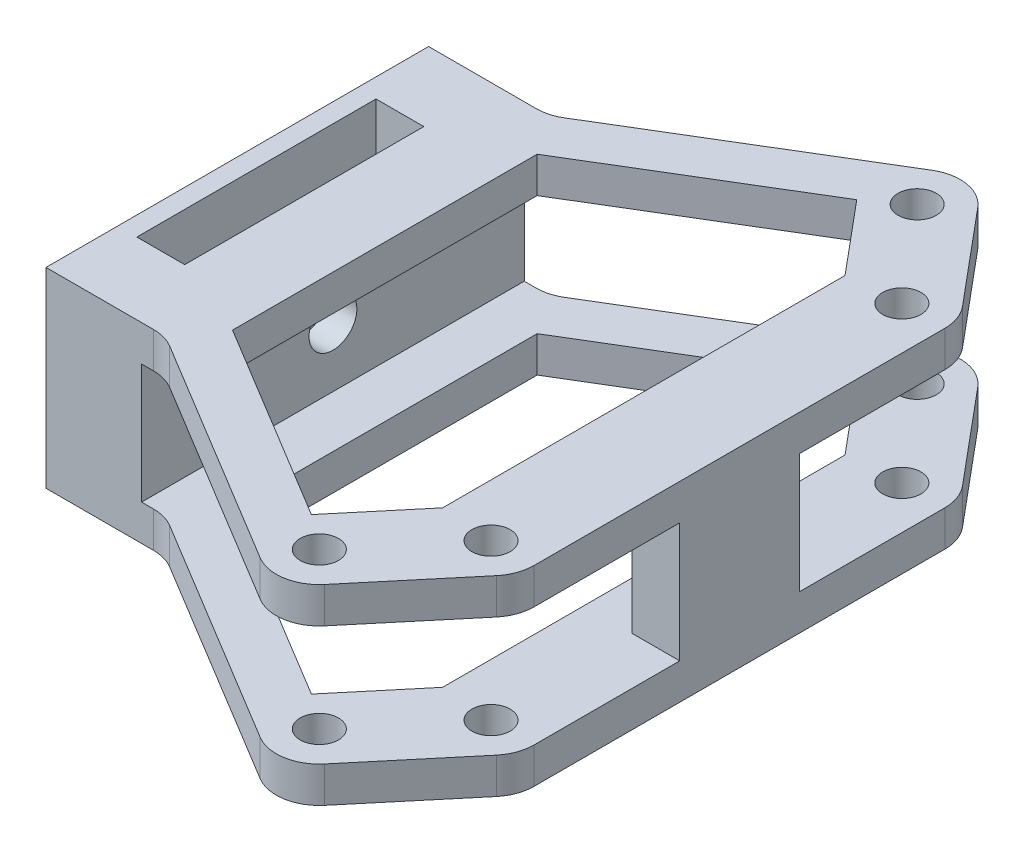
SolidWorks part; units mm, degrees
material "Plain Carbon Steel"
ref_plane "Front Plane" through (0, 0, 0) normal (0, 0, 1) x (1, 0, 0)
ref_plane "Top Plane" through (0, 0, 0) normal (0, 1, 0) x (1, 0, 0)
ref_plane "Right Plane" through (0, 0, 0) normal (1, 0, 0) x (0, 0, -1)
sketch "Frame Profile Sketch" plane through (0, 0, 0) normal (0, 1, 0) x (1, 0, 0)
  line L0 (-1085.7757, 0) -> (53203.0111, 0) construction
  line L1 (0, -1085.7757) -> (0, 53203.0111) construction
  line L2 (25, 40) -> (74.9963, 70.2034)
  line L3 (0, 40) -> (25, 40)
  line L4 (0, 40) -> (0, -40)
  line L5 (0, -40) -> (25, -40)
  line L7 (86.5538, 68.2738) -> (102.9038, 48.7238)
  line L8 (105, 42.95) -> (105, -42.95)
  line L9 (102.9038, -48.7238) -> (86.5538, -68.2738)
  line L10 (74.9963, -70.2034) -> (25, -40)
  arc A0 (102.9038, 48.7238) -> (105, 42.95) centre (96, 42.95) cw
  arc A1 (105, -42.95) -> (102.9038, -48.7238) centre (96, -42.95) cw
  arc A2 (86.5538, 68.2738) -> (74.9963, 70.2034) centre (79.65, 62.5) ccw
  arc A3 (86.5538, -68.2738) -> (74.9963, -70.2034) centre (79.65, -62.5) cw
  dimension "D5" = 9
  dimension "D1" = 80
  dimension "D2" = 25
  dimension "D3" = 40
  dimension "D4" = 105
  dimension "D6" = 16.35
  dimension "D7" = 16.35
  dimension "D8" = 85.9
  dimension "D9" = 42.95
  dimension "D10" = 19.55
  dimension "D11" = 19.55
  dimension "D12" = 25
extrude "Frame Body" add sketch "Frame Profile Sketch" along normal mid plane 40
sketch "Window and Holes Sketch" plane through (0, 0, 0) normal (0, 1, 0) x (1, 0, 0)
  line L0 (0, -1000) -> (0, 49000) construction
  line L1 (74.9963, 70.2034) -> (25, 40) construction
  line L2 (-1000, 0) -> (49000, 0) construction
  line L3 (30.85, 31.8509) -> (30.85, -31.8509)
  line L4 (4, 25) -> (14, 25)
  line L5 (4, 25) -> (4, -25)
  line L6 (4, -25) -> (14, -25)
  line L7 (14, 25) -> (14, -25)
  line L8 (30.85, -31.8509) -> (72.5046, -57.015)
  line L9 (72.5046, -57.015) -> (85, -42.074)
  line L10 (85, -42.074) -> (85, 42.074)
  line L11 (85, 42.074) -> (72.5046, 57.015)
  line L12 (72.5046, 57.015) -> (30.85, 31.8509)
  line L13 (25, -40) -> (74.9963, -70.2034) construction
  line L14 (86.5538, -68.2738) -> (102.9038, -48.7238) construction
  line L15 (102.9038, 48.7238) -> (86.5538, 68.2738) construction
  line L16 (105, -42.95) -> (105, 42.95) construction
  circle A0 centre (79.65, 62.5) radius 4
  circle A1 centre (96, 42.95) radius 4
  circle A2 centre (96, -42.95) radius 4
  circle A3 centre (79.65, -62.5) radius 4
  point P25 (94.7288, 58.4988)
  dimension "D11" = 8
  dimension "D12" = 8
  dimension "D13" = 8
  dimension "D14" = 8
  dimension "D1" = 50
  dimension "D2" = 25
  dimension "D3" = 10
  dimension "D4" = 4
  dimension "D5" = 10
  dimension "D6" = 10
  dimension "D7" = 20
  dimension "D8" = 18
  dimension "D9" = 18
  dimension "D10" = 54.15
extrude "Window and Fixing Holes Cut" cut sketch "Window and Holes Sketch" against normal mid plane 40
sketch "Side Slot Sketch" plane through (0, 0, 0) normal (0, 0, 1) x (1, 0, 0)
  line L0 (-1000, 0) -> (49000, 0) construction
  line L1 (105, 20) -> (105, -20) construction
  line L2 (20, 12.5) -> (95, 12.5)
  line L3 (20, 12.5) -> (20, -12.5)
  line L4 (20, -12.5) -> (95, -12.5)
  line L5 (95, 12.5) -> (95, -12.5)
  dimension "D1" = 25
  dimension "D2" = 12.5
  dimension "D3" = 85
  dimension "D4" = 10
extrude "Side Slot Cut" cut sketch "Side Slot Sketch" against normal mid plane 200
sketch "Top Slot Sketch" plane through (105, 0, 0) normal (1, 0, 0) x (0, 0, -1)
  line L0 (0, -1000) -> (0, 49000) construction
  line L1 (-1000, 0) -> (49000, 0) construction
  line L3 (-71.5, 12.5) -> (-12.5, 12.5)
  line L4 (-71.5, 12.5) -> (-71.5, -12.5)
  line L5 (-71.5, -12.5) -> (-12.5, -12.5)
  line L6 (-12.5, 12.5) -> (-12.5, -12.5)
  line L7 (71.5, 12.5) -> (12.5, 12.5)
  line L8 (71.5, 12.5) -> (71.5, -12.5)
  line L9 (71.5, -12.5) -> (12.5, -12.5)
  line L10 (12.5, 12.5) -> (12.5, -12.5)
  dimension "D1" = 25
  dimension "D2" = 25
  dimension "D3" = 25
  dimension "D4" = 12.5
extrude "Top Slot Cut" cut sketch "Top Slot Sketch" against normal blind 20
sketch "Counterbore Ø24 Sketch" plane through (0, 0, 0) normal (-1, 0, 0) x (0, 0, 1)
  circle A0 centre (0, 0) radius 12
  dimension "D1" = 24
extrude "Counterbore Ø24" cut sketch "Counterbore Ø24 Sketch" against normal blind 3
sketch "Hole Ø10 Sketch" plane through (3, 0, 0) normal (-1, 0, 0) x (0, 0, 1)
  circle A0 centre (0, 0) radius 5
  dimension "D1" = 10
extrude "Hole Ø10" cut sketch "Hole Ø10 Sketch" against normal blind 30
fillet "Corner Fillets R9" radius 9 4 edges at (25, -16.25, -40) (25, 16.25, -40) (25, -16.25, 40) (25, 16.25, 40)
